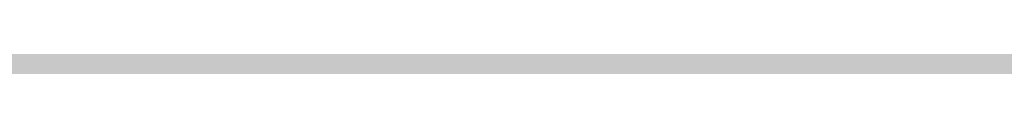
# Model space of a CAD drawing. Units: inches. Extents: x 2091 to 2899, y 967 to 2217.
# Tile 197 of 256: x 2203.18039 to 2203.25707, y 1152.24748 to 1152.2479. Entities that reach past the tile are written whole.
import ezdxf

# ---------------------------------------------------------------- set-up
doc = ezdxf.new("R2010")
doc.units = ezdxf.units.IN
doc.layers.add('A-WALL-PATT', color=141, linetype='Continuous', lineweight=13, true_color=0xadddf7)

msp = doc.modelspace()

# ---------------------------------------------------------------- hatches: boundary and pattern name
at = {"layer": 'A-WALL-PATT'}
h = msp.add_hatch(color=256, dxfattribs=at)
h.dxf.hatch_style = 1
h.paths.add_polyline_path([(2803.143603, 2050.919059), (2203.143603, 2050.919059), (2203.143603, 1090.919059), (2803.143603, 1090.919059)])
h.paths.add_polyline_path([(2635.79885, 1147.540465), (2674.524052, 1147.540465, 0.376086), (2678.529665, 1152.880202), (2678.529665, 1159.556473, 0.333335), (2674.524319, 1163.561846), (2674.524319, 1163.56185), (2674.524319, 1192.93439), (2635.805971, 1192.93439), (2597.087622, 1192.93439), (2597.087622, 1163.561846, 0.333335), (2593.082276, 1159.556473), (2593.082276, 1152.880202, 0.376086), (2597.087889, 1147.540465)], flags=0)
h.paths.add_polyline_path([(2436.010433, 1278.240778, 0.000483), (2435.952643, 1278.215027, -0.001328), (2435.935625, 1278.111693, -0.001711), (2436.11644, 1278.040758, 0.002185)], flags=0)
h.paths.add_polyline_path([(2794.143603, 1143.419059), (2794.143603, 1347.419059), (2543.370171, 1347.419059), (2543.370171, 1351.919059), (2794.143603, 1351.919059), (2794.143603, 1392.713555), (2793.947398, 1392.713555), (2793.947398, 1473.5369), (2794.143603, 1473.5369), (2794.143603, 1531.919059), (2650.143603, 1531.919059), (2650.143603, 1536.419059), (2794.143603, 1536.419059), (2794.143603, 1692.419059), (2609.375609, 1692.419059), (2609.375609, 1644.419059), (2604.875609, 1644.419059), (2604.875609, 1744.919059), (2609.375609, 1744.919059), (2609.375609, 1696.919059), (2794.143603, 1696.919059), (2794.143603, 1780.919059), (2609.643603, 1780.919059), (2493.875609, 1780.919059), (2493.875609, 1785.419059), (2609.643603, 1785.419059), (2794.143603, 1785.419059), (2794.143603, 1847.938821), (2793.951222, 1847.938821), (2793.951222, 1928.762166), (2794.143603, 1928.762166), (2794.143603, 1941.419059), (2614.143603, 1941.419059), (2614.143603, 1821.419059), (2609.643603, 1821.419059), (2609.643603, 1941.419059), (2392.143603, 1941.419059), (2392.143603, 1819.919059), (2387.643603, 1819.919059), (2387.643603, 1941.419059), (2212.143603, 1941.419059), (2212.143603, 1783.919059), (2392.143603, 1783.919059), (2392.143603, 1780.919059), (2212.143603, 1780.919059), (2212.143603, 1629.419059), (2387.643603, 1629.419059), (2387.643603, 1744.919059), (2392.143603, 1744.919059), (2392.143603, 1627.919059), (2317.143603, 1627.919059), (2317.143603, 1551.419059), (2317.143603, 1536.419059), (2459.383591, 1536.419059), (2459.383591, 1602.39648), (2463.883591, 1602.39648), (2463.883591, 1531.919059), (2456.643603, 1531.919059), (2456.643603, 1529.919059), (2452.143603, 1529.919059), (2452.143603, 1531.919059), (2312.643603, 1531.919059), (2312.643603, 1551.419059), (2306.143603, 1551.419059), (2306.143603, 1555.919059), (2308.143603, 1555.919059), (2308.143603, 1551.419059), (2312.643603, 1551.419059), (2312.643603, 1627.919059), (2212.143603, 1627.919059), (2212.143603, 1555.919059), (2270.143603, 1555.919059), (2270.143603, 1551.419059), (2212.143603, 1551.419059), (2212.143603, 1351.919059), (2272.143603, 1351.919059), (2272.143603, 1347.419059), (2212.143603, 1347.419059), (2212.143603, 1275.419059), (2308.143603, 1275.419059), (2308.143603, 1351.919059), (2452.143603, 1351.919059), (2452.143603, 1493.919059), (2456.643603, 1493.919059), (2456.643603, 1347.419059), (2312.643603, 1347.419059), (2312.643603, 1270.919059), (2212.143603, 1270.919059), (2212.143603, 1099.919059), (2281.237523, 1099.919059), (2282.871041, 1110.913803), (2282.008341, 1116.996603), (2278.557741, 1121.420403), (2268.205641, 1128.056203), (2272.087641, 1128.056203), (2273.812941, 1131.927003), (2279.420341, 1134.691903), (2285.027841, 1135.244903), (2287.615841, 1137.456803), (2288.047141, 1138.009803), (2289.341141, 1140.774703), (2291.066541, 1139.668703), (2292.360541, 1135.244903), (2295.379841, 1136.903803), (2296.242541, 1135.797903), (2297.105241, 1133.033003), (2300.124641, 1138.009803), (2303.143941, 1138.009803), (2304.437941, 1135.797903), (2303.143941, 1133.586003), (2306.594641, 1134.691903), (2307.888741, 1133.033003), (2310.908041, 1135.244903), (2313.927441, 1134.138903), (2315.62686, 1132.427102), (2308.320041, 1117.549603), (2290.203841, 1109.807903), (2288.909841, 1103.172103), (2289.272309, 1099.919059), (2434.918227, 1099.919059), (2431.593227, 1124.788059), (2429.930227, 1169.553059), (2430.927185, 1240.519694), (2435.658926, 1238.186126), (2437.135227, 1196.554059), (2438.798227, 1143.973059), (2442.678227, 1111.998059), (2446.558227, 1099.919059), (2794.143603, 1099.919059), (2794.143603, 1138.919059), (2548.032447, 1138.919059), (2548.032447, 1143.419059), (2548.032447, 1148.819059), (2546.668457, 1148.031559), (2528.685692, 1179.178622, 0.256256), (2512.032447, 1148.819059), (2512.032447, 1143.419059), (2512.032447, 1138.919059), (2507.532447, 1138.919059), (2507.532447, 1143.419059), (2507.532447, 1148.819059, 0.256256), (2490.879202, 1179.178622), (2472.896437, 1148.031559), (2471.532447, 1148.819059), (2471.532447, 1143.419059), (2467.032447, 1143.419059), (2467.032447, 1269.945786, 0.039061), (2460.909987, 1273.580059), (2467.032447, 1273.580059), (2467.032447, 1286.325364, 0.014511), (2465.216194, 1286.761905), (2467.032447, 1287.052576), (2467.032447, 1323.419059), (2471.532447, 1323.419059), (2471.532447, 1148.819059), (2489.532447, 1179.995973), (2490.896437, 1179.208473), (2490.879202, 1179.178622, -0.256256), (2507.532447, 1148.819059), (2507.532447, 1143.419059), (2512.032447, 1143.419059), (2512.032447, 1148.819059, -0.256256), (2528.685692, 1179.178622), (2528.668457, 1179.208473), (2530.032447, 1179.995973), (2548.032447, 1148.819059), (2548.032447, 1143.419059)], flags=16)
h.paths.add_polyline_path([(2607.768546, 1200.945083), (2607.768546, 1265.030625), (2597.087622, 1281.052011), (2619.784585, 1281.052011), (2627.795278, 1337.12686), (2635.79885, 1337.12686), (2643.816663, 1337.12686), (2651.827356, 1281.052011), (2674.524319, 1281.052011), (2663.843395, 1265.030625), (2663.843395, 1200.945083), (2635.805971, 1200.945083)], flags=0)
edge = h.paths.add_edge_path(flags=0)
edge.add_ellipse((13303.896215, 1272.998725), major_axis=(-10595.31304, 0.000001), ratio=0.842303870086, start_angle=0.6282372191, end_angle=0.6465540999, ccw=False)
edge.add_ellipse((2711.70045, 1156.852678), major_axis=(2.219769, 0), ratio=0.84230387, start_angle=111.535244, end_angle=180.628237, ccw=False)
edge.add_ellipse((13303.156292, 1272.998725), major_axis=(-10593.026306, 0), ratio=0.842303869544, start_angle=0.5282714718, end_angle=0.6465540971, ccw=False)
edge.add_line((2710.764596, 1175.333295), (2710.129986, 1175.333295))
edge.add_ellipse((2710.129986, 1176.579775), major_axis=(1.479846, 0), ratio=0.84230387, start_angle=180, end_angle=270, ccw=False)
edge.add_line((2708.65014, 1176.579775), (2708.65014, 1200.782914))
edge.add_ellipse((2710.129986, 1200.782914), major_axis=(1.479846, 0), ratio=0.84230387, start_angle=90, end_angle=180, ccw=False)
edge.add_line((2710.129986, 1202.029394), (2710.465075, 1202.029394))
edge.add_ellipse((13303.156292, 1272.998725), major_axis=(-10593.026306, 0), ratio=0.842303869544, start_angle=-0.0902290886, end_angle=0.3838667788, ccw=False)
edge.add_ellipse((2710.129986, 1290.927031), major_axis=(-1.479846, 0), ratio=0.84230387, start_angle=0, end_angle=90, ccw=False)
edge.add_line((2708.65014, 1290.927031), (2708.65014, 1315.13017))
edge.add_ellipse((2710.129986, 1315.13017), major_axis=(-1.479846, 0), ratio=0.84230387, start_angle=-90, end_angle=0, ccw=False)
edge.add_line((2710.129986, 1316.37665), (2710.706314, 1316.37665))
edge.add_ellipse((3238.40172, 1296.289566), major_axis=(528.234, 0), ratio=0.8423038695, start_angle=176.34957241, end_angle=177.82004969, ccw=False)
edge.add_ellipse((2775.063043, 1071.450696), major_axis=(313.307761, 0), ratio=0.8423038695, start_angle=102.12596555, end_angle=103.78052899, ccw=False)
edge.add_ellipse((2775.063043, 1078.305698), major_axis=(-305.302891, 0), ratio=0.8423038695, start_angle=-79.790461, end_angle=-77.55537271, ccw=False)
edge.add_ellipse((2695.141767, 1541.975383), major_axis=(-250.960216, 0), ratio=0.8423038695, start_angle=99.25656601, end_angle=102.55493264)
edge.add_line((2741.410326, 1334.214255), (2747.132545, 1337.378477))
edge.add_ellipse((2747.538616, 1336.857478), major_axis=(-0.739923, 0), ratio=0.8423039, start_angle=270, end_angle=307.93313, ccw=False)
edge.add_ellipse((2747.538616, 1336.857478), major_axis=(-0.739923, 0), ratio=0.8423039, start_angle=232.06687, end_angle=270, ccw=False)
edge.add_line((2747.944687, 1337.378477), (2753.666906, 1334.214255))
edge.add_ellipse((2799.935466, 1541.975383), major_axis=(250.960216, 0), ratio=0.8423038695, start_angle=257.44506736, end_angle=260.74343399)
edge.add_ellipse((2720.014189, 1078.305698), major_axis=(305.302891, 0), ratio=0.8423038695, start_angle=77.55537271, end_angle=79.790461, ccw=False)
edge.add_ellipse((2720.014189, 1071.450696), major_axis=(-313.307761, 0), ratio=0.8423038695, start_angle=256.21947101, end_angle=257.87403445, ccw=False)
edge.add_ellipse((2256.675512, 1296.289566), major_axis=(-528.234, 0), ratio=0.8423038695, start_angle=182.17995031, end_angle=183.65042759, ccw=False)
edge.add_line((2784.370918, 1316.37665), (2784.947247, 1316.37665))
edge.add_ellipse((2784.947247, 1315.13017), major_axis=(1.479846, 0), ratio=0.84230387, start_angle=0, end_angle=90, ccw=False)
edge.add_line((2786.427093, 1315.13017), (2786.427093, 1290.927031))
edge.add_ellipse((2784.947247, 1290.927031), major_axis=(1.479846, 0), ratio=0.84230387, start_angle=270, end_angle=360, ccw=False)
edge.add_ellipse((-7808.07906, 1272.998725), major_axis=(10593.026306, 0), ratio=0.842303869544, start_angle=-0.3838667788, end_angle=0.0902290886, ccw=False)
edge.add_line((2784.612157, 1202.029394), (2784.947247, 1202.029394))
edge.add_ellipse((2784.947247, 1200.782914), major_axis=(1.479846, 0), ratio=0.84230387, start_angle=0, end_angle=90, ccw=False)
edge.add_line((2786.427093, 1200.782914), (2786.427093, 1176.579775))
edge.add_ellipse((2784.947247, 1176.579775), major_axis=(-1.479846, 0), ratio=0.84230387, start_angle=90, end_angle=180, ccw=False)
edge.add_line((2784.947247, 1175.333295), (2784.312636, 1175.333295))
edge.add_ellipse((-7808.07906, 1272.998725), major_axis=(10593.026306, 0), ratio=0.842303869544, start_angle=-0.6186431963, end_angle=-0.5282714718, ccw=False)
edge.add_ellipse((2783.376783, 1156.852678), major_axis=(-2.219769, 0), ratio=0.84230387, start_angle=179.371763, end_angle=248.464757, ccw=False)
edge.add_ellipse((-7808.818983, 1272.998725), major_axis=(-10595.31304, 0.000004), ratio=0.842303865762, start_angle=179.3534459226, end_angle=179.3717628034, ccw=False)
edge.add_ellipse((2780.297303, 1153.500793), major_axis=(-5.246426, 0), ratio=0.84230387, start_angle=90, end_angle=179.353446, ccw=False)
edge.add_line((2780.297303, 1149.081708), (2714.77993, 1149.081708))
edge.add_ellipse((2714.77993, 1153.500793), major_axis=(5.246426, 0), ratio=0.84230387, start_angle=180.646554, end_angle=270, ccw=False)
edge = h.paths.add_edge_path(flags=0)
edge.add_line((2718.187367, 1151.007833), (2718.187367, 1170.472364))
edge.add_ellipse((2721.14706, 1170.472364), major_axis=(-2.959692, 0), ratio=0.84230387, start_angle=-90, end_angle=0, ccw=False)
edge.add_line((2721.14706, 1172.965324), (2773.930173, 1172.965324))
edge.add_ellipse((2773.930173, 1170.472364), major_axis=(-2.959692, 0), ratio=0.84230387, start_angle=180, end_angle=270, ccw=False)
edge.add_line((2776.889865, 1170.472364), (2776.889865, 1151.007833))
edge.add_line((2776.889865, 1151.007833), (2718.187367, 1151.007833))
edge = h.paths.add_edge_path(flags=0)
edge.add_line((2718.187367, 1180.23415), (2718.187367, 1199.057834))
edge.add_ellipse((2747.538616, 1320.39864), major_axis=(147.017924, 0), ratio=0.8423038695, start_angle=256.40186531, end_angle=283.59813469)
edge.add_line((2776.889865, 1199.057834), (2776.889865, 1180.23415))
edge.add_ellipse((2747.538616, 1301.574956), major_axis=(147.017924, 0), ratio=0.8423038695, start_angle=256.40186531, end_angle=283.59813469, ccw=False)
edge = h.paths.add_edge_path(flags=0)
edge.add_ellipse((13303.156292, 1272.998725), major_axis=(-10591.54646, 0), ratio=0.842303869555, start_angle=0.0555943135, end_angle=0.3777641939, ccw=False)
edge.add_line((2711.616859, 1262.72171), (2715.667408, 1249.495396))
edge.add_ellipse((6413.891963, 1241.691919), major_axis=(-3698.236159, 0), ratio=0.84230386955, start_angle=-0.120897369, end_angle=0.364076349)
edge.add_line((2715.761038, 1218.192455), (2711.934307, 1203.167361))
edge = h.paths.add_edge_path(flags=0)
edge.add_line((2718.187367, 1251.074566), (2716.002485, 1267.450435))
edge.add_ellipse((2742.151175, 1202.18954), major_axis=(81.772585, 0), ratio=0.84230387, start_angle=94.27742096, end_angle=111.8349538, ccw=False)
edge.add_line((2737.009748, 1270.930626), (2758.067484, 1270.930626))
edge.add_ellipse((2752.926058, 1202.18954), major_axis=(81.772585, 0), ratio=0.84230387, start_angle=68.1650462, end_angle=85.72257904, ccw=False)
edge.add_line((2779.074747, 1267.450435), (2776.889865, 1251.074566))
edge.add_ellipse((2750.338059, 1187.885356), major_axis=(79.579664, 0), ratio=0.84230387, start_angle=67.20808512, end_angle=85.1299304)
edge.add_line((2756.034656, 1254.743656), (2739.042576, 1254.743656))
edge.add_ellipse((2744.739174, 1187.885356), major_axis=(79.579664, 0), ratio=0.84230387, start_angle=94.8700696, end_angle=112.79191488)
edge = h.paths.add_edge_path(flags=0)
edge.add_line((2783.142926, 1203.167361), (2779.316194, 1218.192455))
edge.add_ellipse((-918.81473, 1241.691919), major_axis=(3698.236159, 0), ratio=0.84230386955, start_angle=-0.364076349, end_angle=0.120897369)
edge.add_line((2779.409825, 1249.495396), (2783.460373, 1262.72171))
edge.add_ellipse((-7808.07906, 1272.998725), major_axis=(-10591.54646, 0), ratio=0.84230386954, start_angle=179.6222358061, end_angle=179.9444056865, ccw=False)
edge = h.paths.add_edge_path(flags=0)
edge.add_ellipse((2734.200892, 1286.69044), major_axis=(-0.356609, 6.340078), ratio=0.60383358, start_angle=89.0020143, end_angle=253.657408, ccw=False)
edge.add_line((2730.369001, 1286.541806), (2730.369001, 1301.35198))
edge.add_line((2730.369001, 1301.35198), (2735.913311, 1305.214803))
edge.add_ellipse((2736.384917, 1304.734561), major_axis=(0.739923, 0), ratio=0.8423039, start_angle=90, end_angle=134.480211, ccw=False)
edge.add_line((2736.384917, 1305.357801), (2738.032783, 1305.357801))
edge.add_line((2738.032783, 1305.357801), (2738.032783, 1307.707927))
edge.add_ellipse((2794.201642, 1307.707927), major_axis=(56.168859, 0), ratio=0.84230387, start_angle=150.5614304, end_angle=180, ccw=False)
edge.add_ellipse((2700.875591, 1307.707927), major_axis=(-56.168859, 0), ratio=0.84230387, start_angle=180, end_angle=209.4385696, ccw=False)
edge.add_line((2757.04445, 1307.707927), (2757.04445, 1305.357801))
edge.add_line((2757.04445, 1305.357801), (2758.692316, 1305.357801))
edge.add_ellipse((2758.692316, 1304.734561), major_axis=(-0.739923, 0), ratio=0.8423039, start_angle=225.519789, end_angle=270, ccw=False)
edge.add_line((2759.163922, 1305.214803), (2764.708231, 1301.35198))
edge.add_line((2764.708231, 1301.35198), (2764.708231, 1286.541806))
edge.add_ellipse((2760.87634, 1286.69044), major_axis=(0.356609, 6.340078), ratio=0.60383358, start_angle=106.342592, end_angle=270.9979857, ccw=False)
edge.add_line((2757.04445, 1285.79709), (2757.04445, 1307.707927))
edge.add_ellipse((2700.875591, 1307.707927), major_axis=(-56.168859, 0), ratio=0.84230387, start_angle=180, end_angle=209.4385696)
edge.add_ellipse((2794.201642, 1307.707927), major_axis=(56.168859, 0), ratio=0.84230387, start_angle=150.5614304, end_angle=180)
edge.add_line((2738.032783, 1307.707927), (2738.032783, 1285.79709))
h.paths.add_polyline_path([(2417.812273, 1104.449704), (2413.492273, 1102.529704), (2410.612273, 1103.969704), (2409.172273, 1106.369704), (2407.252273, 1107.329704), (2406.292273, 1109.729704), (2405.332273, 1114.049704), (2405.332273, 1117.889704), (2406.292273, 1120.129704), (2407.252273, 1119.809704), (2408.848322, 1118.327658), (2410.173945, 1119.42417), (2410.211273, 1120.405704), (2411.040731, 1121.419054), (2410.699273, 1119.858704), (2410.173945, 1119.42417), (2410.088452, 1117.176109), (2411.132836, 1116.206324), (2413.972273, 1119.329704), (2416.852273, 1120.769704), (2416.869721, 1120.798784), (2417.035071, 1119.405116), (2417.896213, 1118.143384), (2418.292273, 1118.369704), (2419.544447, 1120.039269), (2419.360915, 1118.387487), (2419.032108, 1119.356151), (2418.398939, 1118.511926), (2419.252273, 1114.529704), (2418.794091, 1107.198795)], flags=0)
h.paths.add_polyline_path([(2508.870171, 1347.419059), (2508.370171, 1347.419059), (2508.370171, 1351.919059), (2508.870171, 1351.919059)], flags=0)
h.paths.add_polyline_path([(2473.370171, 1347.419059), (2472.370171, 1347.419059), (2467.870171, 1347.419059), (2467.870171, 1455.419059), (2472.370171, 1455.419059), (2472.370171, 1352.419059), (2473.370171, 1352.419059)], flags=0)
h.paths.add_polyline_path([(2352.106244, 1217.446197), (2349.226244, 1218.886197), (2347.786244, 1221.286197), (2345.866244, 1222.246197), (2344.906244, 1224.646197), (2343.946244, 1228.966197), (2343.946244, 1232.806197), (2344.906244, 1235.046197), (2345.866244, 1234.726197), (2347.462293, 1233.244152), (2348.787916, 1234.340663), (2348.825244, 1235.322197), (2349.654702, 1236.335547), (2349.313244, 1234.775197), (2348.787916, 1234.340663), (2348.702423, 1232.092603), (2349.746807, 1231.122817), (2352.586244, 1234.246197), (2355.466244, 1235.686197), (2355.483692, 1235.715277), (2355.649043, 1234.321609), (2356.510185, 1233.059877), (2356.906244, 1233.286197), (2358.158418, 1234.955762), (2357.974887, 1233.30398), (2357.646079, 1234.272644), (2357.012911, 1233.428419), (2357.866244, 1229.446197), (2357.408062, 1222.115288), (2356.426244, 1219.366197)], flags=0)
h.paths.add_polyline_path([(2348.2968, 1112.22442), (2347.0138, 1112.31042), (2345.5298, 1114.12742), (2345.7318, 1115.85842), (2346.8118, 1116.98242), (2346.8118, 1114.64642), (2345.8668, 1114.21442), (2346.8798, 1114.30042)], flags=0)
h.paths.add_polyline_path([(2347.0138, 1110.92642), (2346.2718, 1110.49342), (2346.6098, 1111.18642)], flags=0)
h.paths.add_polyline_path([(2345.8668, 1118.19442), (2345.5298, 1117.32942), (2343.7078, 1118.02142), (2344.3828, 1118.62642)], flags=0)
h.paths.add_polyline_path([(2346.6768, 1109.28242), (2346.0698, 1108.07142), (2345.8668, 1110.06142)], flags=0)
h.paths.add_polyline_path([(2345.0568, 1119.75142), (2343.6398, 1119.75142), (2343.9778, 1121.13542)], flags=0)
h.paths.add_polyline_path([(2345.2598, 1116.55042), (2345.1248, 1115.85842), (2344.9218, 1115.68542), (2344.7198, 1116.37742)], flags=0)
h.paths.add_polyline_path([(2345.6648, 1112.31042), (2345.4618, 1111.53242), (2344.0448, 1111.96442), (2344.6518, 1112.57042)], flags=0)
h.paths.add_polyline_path([(2345.1918, 1113.34942), (2344.4498, 1113.86842), (2344.7198, 1114.38742)], flags=0)
h.paths.add_polyline_path([(2344.6518, 1116.80942), (2344.1798, 1115.68542), (2344.6518, 1115.33942), (2343.9098, 1114.90642), (2343.0328, 1115.94442), (2343.6398, 1116.46342)], flags=0)
h.paths.add_polyline_path([(2345.8668, 1106.68642), (2344.9898, 1105.56242), (2344.5168, 1106.60042)], flags=0)
h.paths.add_polyline_path([(2344.8548, 1110.06142), (2344.5168, 1109.28242), (2344.1128, 1109.71542)], flags=0)
h.paths.add_polyline_path([(2344.0448, 1113.52242), (2343.4378, 1113.08942), (2342.7628, 1113.95442)], flags=0)
h.paths.add_polyline_path([(2344.3148, 1111.01242), (2342.9648, 1110.32042), (2342.9648, 1111.09942)], flags=0)
h.paths.add_polyline_path([(2345.1248, 1104.69742), (2344.5848, 1103.74542), (2344.4498, 1104.26442)], flags=0)
h.paths.add_polyline_path([(2342.8298, 1121.22242), (2341.7498, 1120.53042), (2340.5358, 1121.04942), (2340.1308, 1121.82842), (2340.6708, 1122.95242), (2341.1428, 1121.82842), (2341.6148, 1122.00142)], flags=0)
h.paths.add_polyline_path([(2342.9648, 1119.75142), (2343.0328, 1118.45342), (2342.0878, 1118.02142), (2342.0198, 1119.49142)], flags=0)
h.paths.add_polyline_path([(2342.6948, 1116.89642), (2341.9528, 1116.63642), (2342.0198, 1117.32942)], flags=0)
h.paths.add_polyline_path([(2343.0328, 1112.22442), (2342.0198, 1111.79142), (2341.5478, 1112.22442), (2342.3578, 1113.34942)], flags=0)
h.paths.add_polyline_path([(2343.7748, 1104.43742), (2342.6278, 1102.88042), (2342.6948, 1104.61042), (2343.4378, 1105.12942)], flags=0)
h.paths.add_polyline_path([(2342.0198, 1115.07942), (2340.8058, 1115.51242), (2340.9408, 1116.37742)], flags=0)
h.paths.add_polyline_path([(2341.4808, 1120.09742), (2341.4808, 1119.40542), (2341.0758, 1119.57842), (2341.1428, 1120.09742)], flags=0)
h.paths.add_polyline_path([(2341.8178, 1114.47342), (2340.9408, 1113.08942), (2340.8058, 1114.56042)], flags=0)
h.paths.add_polyline_path([(2341.1428, 1118.54042), (2340.9408, 1116.98242), (2339.0508, 1117.67542), (2339.0508, 1118.62642)], flags=0)
h.paths.add_polyline_path([(2342.6948, 1101.66842), (2341.9528, 1101.84142), (2342.5598, 1102.36142)], flags=0)
h.paths.add_polyline_path([(2340.3328, 1119.66542), (2338.4438, 1119.57842), (2337.9038, 1120.35742), (2339.6578, 1120.61642)], flags=0)
h.paths.add_polyline_path([(2340.3328, 1115.33942), (2340.0628, 1113.69542), (2339.3878, 1115.33942)], flags=0)
h.paths.add_polyline_path([(2341.8178, 1103.83142), (2341.5478, 1102.88042), (2341.1428, 1103.65842)], flags=0)
h.paths.add_polyline_path([(2339.0508, 1122.86642), (2337.2958, 1121.82842), (2337.0938, 1123.12542), (2337.7688, 1123.81842)], flags=0)
h.paths.add_polyline_path([(2339.1178, 1121.74142), (2338.8478, 1121.22242), (2338.1738, 1121.04942), (2338.3758, 1121.56842)], flags=0)
h.paths.add_polyline_path([(2339.1858, 1119.31942), (2338.6458, 1118.71342), (2338.2408, 1118.10742), (2338.2408, 1118.88642)], flags=0)
h.paths.add_polyline_path([(2341.1428, 1101.92842), (2340.6028, 1101.23642), (2340.0628, 1101.84142), (2340.6028, 1102.36142)], flags=0)
h.paths.add_polyline_path([(2337.6338, 1117.76142), (2336.6208, 1118.28042), (2337.2958, 1118.97242)], flags=0)
h.paths.add_polyline_path([(2336.8238, 1119.57842), (2334.7988, 1118.97242), (2335.2038, 1120.35742), (2336.5538, 1120.87642)], flags=0)
h.paths.add_polyline_path([(2339.1178, 1100.45742), (2337.3638, 1100.54342), (2336.7558, 1101.23642)], flags=0)
h.paths.add_polyline_path([(2336.3508, 1122.43342), (2336.0138, 1121.91442), (2334.9338, 1122.43342), (2334.5288, 1123.47142), (2335.7438, 1122.77942)], flags=0)
h.paths.add_polyline_path([(2334.7318, 1120.87642), (2334.2588, 1120.35742), (2334.0568, 1120.78942), (2334.5968, 1121.30842)], flags=0)
h.paths.add_polyline_path([(2334.4618, 1122.17442), (2332.5718, 1121.30842), (2331.3568, 1122.17442), (2332.0998, 1122.86642)], flags=0)
h.paths.add_polyline_path([(2334.2588, 1118.54042), (2333.3818, 1118.45342), (2333.6518, 1119.31942)], flags=0)
h.paths.add_polyline_path([(2335.5418, 1102.27442), (2334.1918, 1102.62042), (2335.2718, 1103.31242)], flags=0)
h.paths.add_polyline_path([(2332.7068, 1119.66542), (2331.6948, 1120.44342), (2332.5048, 1120.78942)], flags=0)
h.paths.add_polyline_path([(2334.7318, 1101.14942), (2333.5168, 1101.58242), (2333.9888, 1101.75542)], flags=0)
h.paths.add_polyline_path([(2332.6398, 1116.63642), (2331.0868, 1116.29042), (2331.9648, 1118.19442)], flags=0)
h.paths.add_polyline_path([(2330.7498, 1121.56842), (2330.2768, 1120.27042), (2328.5228, 1119.31942), (2328.9948, 1121.04942)], flags=0)
h.paths.add_polyline_path([(2330.7498, 1118.62642), (2330.0078, 1117.50242), (2329.8728, 1118.02142)], flags=0)
h.paths.add_polyline_path([(2332.0998, 1102.36142), (2330.5468, 1102.01442), (2331.6948, 1102.96642)], flags=0)
h.paths.add_polyline_path([(2329.5348, 1113.60842), (2329.0628, 1112.31042), (2328.5898, 1113.34942)], flags=0)
h.paths.add_polyline_path([(2328.3878, 1117.84842), (2327.5098, 1116.55042), (2327.1728, 1117.76142)], flags=0)
h.paths.add_polyline_path([(2329.7378, 1106.51342), (2329.5348, 1105.30242), (2328.2528, 1106.08142)], flags=0)
h.paths.add_polyline_path([(2328.6578, 1114.38742), (2328.0498, 1114.12742), (2328.3198, 1114.90642)], flags=0)
h.paths.add_polyline_path([(2328.3198, 1112.22442), (2327.1058, 1112.13742), (2326.7008, 1112.65642)], flags=0)
h.paths.add_polyline_path([(2326.9028, 1115.25242), (2326.7008, 1114.12742), (2325.2158, 1113.60842), (2326.0928, 1115.33942)], flags=0)
h.paths.add_polyline_path([(2326.6328, 1108.33042), (2326.0928, 1107.37942), (2325.8908, 1108.50342), (2326.4978, 1109.10942)], flags=0)
h.paths.add_polyline_path([(2615.143603, 1531.919059), (2609.643603, 1531.919059), (2609.643603, 1620.419059), (2614.143603, 1620.419059), (2614.143603, 1536.419059), (2615.143603, 1536.419059)], flags=0)
h.paths.add_polyline_path([(2545.143603, 1563.419059), (2464.143603, 1563.419059), (2464.143603, 1632.419059), (2509.143603, 1632.419059), (2509.143603, 1627.919059), (2509.143603, 1603.919059), (2468.643603, 1603.919059), (2468.643603, 1567.919059), (2540.643603, 1567.919059), (2540.643603, 1591.919059), (2545.143603, 1591.919059)], flags=0)
h.paths.add_polyline_path([(2388.969048, 1549.985735), (2357.434181, 1549.985735), (2357.434181, 1623.360778), (2399.362777, 1623.360778), (2435.689465, 1623.360778), (2435.592547, 1602.559273), (2435.592547, 1602.39648), (2388.969048, 1602.39648)], flags=0)
h.paths.add_polyline_path([(2388.880628, 1555.809151), (2374.904429, 1555.809151), (2374.904429, 1600.571564), (2374.904429, 1615.457645), (2406.350877, 1615.457645), (2406.350877, 1618.939431), (2412.174293, 1615.457645), (2406.350877, 1611.97586), (2406.350877, 1615.457645), (2388.880628, 1615.457645)], flags=0)
h.paths.add_polyline_path([(2568.875609, 1644.419059), (2453.375609, 1644.419059), (2453.375609, 1785.419059), (2457.875609, 1785.419059), (2457.875609, 1648.919059), (2568.875609, 1648.919059)], flags=0)
h.paths.add_polyline_path([(2212.143603, 1945.919059), (2212.143603, 2041.919059), (2794.143603, 2041.919059), (2794.143603, 1945.919059)], flags=16)
h.paths.add_polyline_path([(2271.082728, 1964.317238), (2776.852968, 1964.317238), (2776.852968, 2037.169623), (2271.082728, 2037.169623)], flags=8)
h.paths.add_polyline_path([(2380.649285, 1536.824144), (2461.040809, 1536.824144), (2461.040809, 1554.652587), (2380.649285, 1554.652587)], flags=8)
h.paths.add_polyline_path([(2240.755709, 1609.725451), (2309.185829, 1609.725451), (2309.185829, 1617.698204), (2240.755709, 1617.698204)], flags=8)
h.paths.add_polyline_path([(2212.677255, 1313.504102), (2282.59152, 1313.504102), (2282.59152, 1322.745239), (2212.677255, 1322.745239)], flags=8)
h.paths.add_polyline_path([(2457.111976, 1114.778574), (2558.481581, 1114.778574), (2558.481581, 1142.219682), (2457.111976, 1142.219682)], flags=8)
h.paths.add_polyline_path([(2473.442337, 1273.010067), (2604.641226, 1273.010067), (2604.641226, 1318.346935), (2473.442337, 1318.346935)], flags=8)
h.paths.add_polyline_path([(2638.876302, 1626.977432), (2684.250367, 1627.976738), (2684.038483, 1637.597494), (2638.664417, 1636.598188)], flags=8)
h.paths.add_polyline_path([(2537.590554, 1453.793447), (2628.389547, 1453.793447), (2628.389547, 1475.344811), (2537.590554, 1475.344811)], flags=8)
h.paths.add_polyline_path([(2504.137638, 1714.632397), (2554.647187, 1714.632397), (2554.647187, 1730.237712), (2504.137638, 1730.237712)], flags=8)
h.paths.add_polyline_path([(2487.501181, 1575.651872), (2535.097121, 1575.651872), (2535.097121, 1598.377646), (2487.501181, 1598.377646)], flags=8)
h.paths.add_polyline_path([(2709.0994, 1735.710278), (2740.016601, 1735.710278), (2740.016601, 1749.937641), (2709.0994, 1749.937641)], flags=8)
h.paths.add_polyline_path([(2442.438424, 1792.171657), (2564.728835, 1792.171657), (2564.728835, 1842.000163), (2442.438424, 1842.000163)], flags=8)
h.paths.add_polyline_path([(2655.815801, 1809.644076), (2789.520142, 1806.693796), (2790.084977, 1832.291638), (2656.380635, 1835.241918)], flags=8)
h.paths.add_polyline_path([(2234.842697, 1797.720143), (2368.592851, 1794.768852), (2369.160718, 1820.504132), (2235.410564, 1823.455423)], flags=8)
h.paths.add_polyline_path([(2245.138466, 1644.006335), (2398.427733, 1640.6239), (2398.994842, 1666.32482), (2245.705575, 1669.707255)], flags=8)
h.paths.add_polyline_path([(2306.142847, 1431.168519), (2413.768314, 1428.793687), (2414.333148, 1454.391529), (2306.707682, 1456.76636)], flags=8)
h.paths.add_polyline_path([(2306.834582, 1458.233145), (2393.380484, 1456.323449), (2393.932808, 1481.354358), (2307.386907, 1483.264054)], flags=8)

doc.saveas('drawing.dxf')
